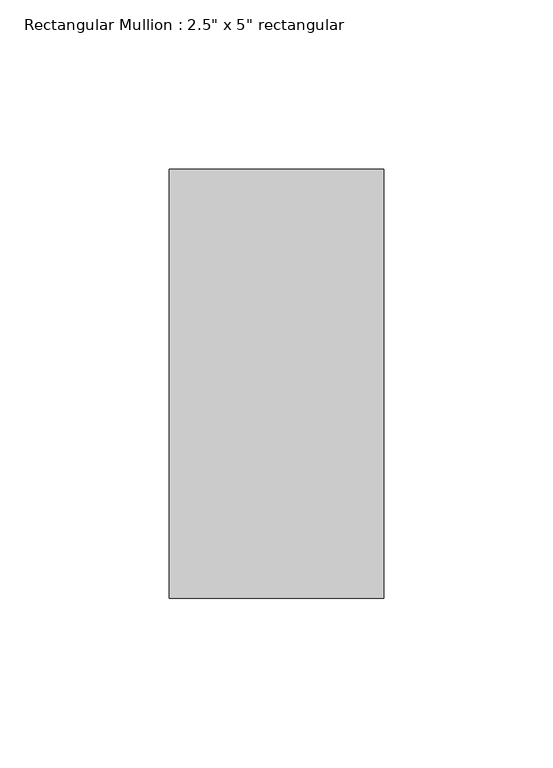
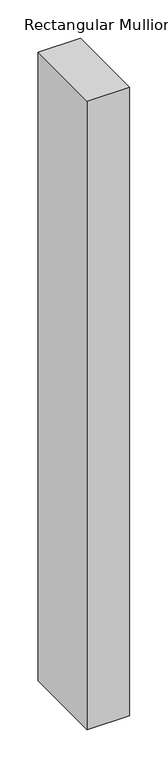
"""IFC4 building model written with IfcOpenShell, lengths in millimetres: member geometry."""

from ifc_helpers import new_model, si_unit, frame, origin, place, context, project, spatial, polyline, outline, extrude, source, transform, mapped, element, save


def member_30308bf7(model_context):
    return source(origin(), model_context, "Body", "SweptSolid", [
        extrude(outline(polyline([(0.0, 63.5), (0.0, -63.5), (-63.5, -63.5), (-63.5, 63.5), (0.0, 63.5)])), frame((0.0, 0.0, -996.9500001), z_axis=(0.0, 0.0, 1.0), x_axis=(1.0, 0.0, 0.0)), (0.0, 0.0, 1.0), 996.9500001),
    ])


if __name__ == "__main__":
    model = new_model("IFC4")
    model_context = context("Model", 3, world=origin())
    ifc_project = project(units=[si_unit("LENGTHUNIT", "METRE", prefix="MILLI")], contexts=[model_context])
    site = spatial("IfcSite", under=ifc_project)
    building = spatial("IfcBuilding", under=site)
    placement = place(None, origin())
    member_shape = member_30308bf7(model_context)
    element("IfcMember", 1, ObjectType="Rectangular Mullion : 2.5\" x 5\" rectangular", at=placement, inside=building, context=model_context, shape_type="MappedRepresentation", body=[
        mapped(member_shape, transform((0.0, 0.0, 0.0), x_axis=(1.0, 0.0, 0.0), y_axis=(0.0, 1.0, 0.0), z_axis=(0.0, 0.0, 1.0))),
    ])
    save(model, "model.ifc")

# Revit data of these elements
# Type "Rectangular Mullion : 2.5\" x 5\" rectangular"
#   built-in parameter 1007304 = 0.416667 (stored number, unit not read)
#   built-in parameter 1007301 = 0.104167 (stored number, unit not read)
#   built-in parameter 1007300 = 0.104167 (stored number, unit not read)
# Element 1 (IfcMember, "Rectangular Mullion : 2.5\" x 5\" rectangular")
#   Materials on its faces: "Aluminum"
# Materials
#   "Aluminum": class "Metal", colour RGB 247 247 247, transparency 0, Description = "Aluminum 6061", Cost = 0
